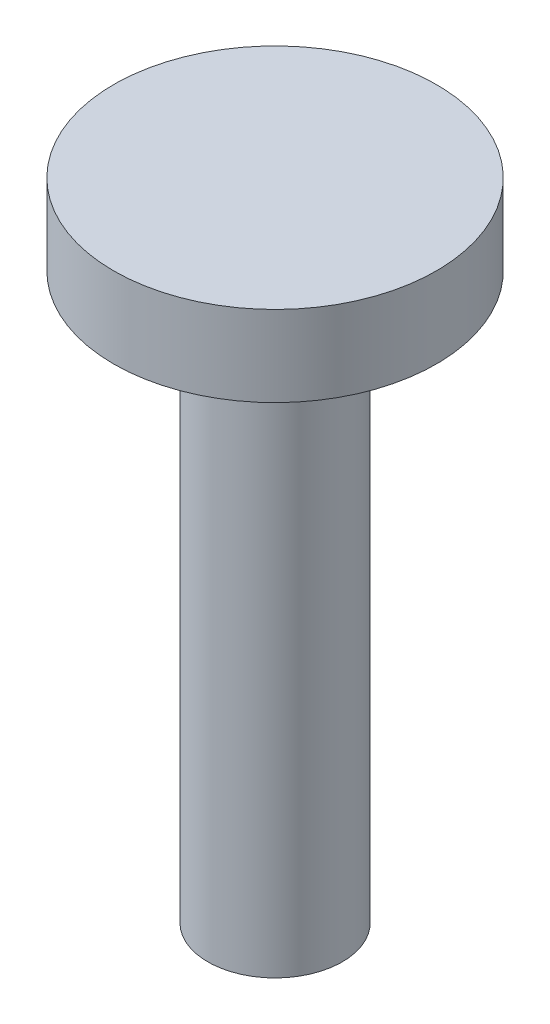
ISO-10303-21;
HEADER;
FILE_DESCRIPTION(('STEP AP214'),'2;1');
FILE_NAME('part.step','',(''),(''),'','','');
FILE_SCHEMA(('AUTOMOTIVE_DESIGN { 1 0 10303 214 1 1 1 1 }'));
ENDSEC;
DATA;
#1=APPLICATION_CONTEXT('core data for automotive mechanical design processes');
#2=APPLICATION_PROTOCOL_DEFINITION('international standard','automotive_design',2000,#1);
#3=PRODUCT_CONTEXT('',#1,'mechanical');
#4=PRODUCT('Part','Part','',(#3));
#5=PRODUCT_RELATED_PRODUCT_CATEGORY('part','',(#4));
#6=PRODUCT_DEFINITION_FORMATION('','',#4);
#7=PRODUCT_DEFINITION_CONTEXT('part definition',#1,'design');
#8=PRODUCT_DEFINITION('design','',#6,#7);
#9=PRODUCT_DEFINITION_SHAPE('','',#8);
#10=(LENGTH_UNIT() NAMED_UNIT(*) SI_UNIT(.MILLI.,.METRE.));
#11=(NAMED_UNIT(*) PLANE_ANGLE_UNIT() SI_UNIT($,.RADIAN.));
#12=(NAMED_UNIT(*) SI_UNIT($,.STERADIAN.) SOLID_ANGLE_UNIT());
#13=UNCERTAINTY_MEASURE_WITH_UNIT(LENGTH_MEASURE(1.E-05),#10,'distance_accuracy_value','');
#14=(GEOMETRIC_REPRESENTATION_CONTEXT(3) GLOBAL_UNCERTAINTY_ASSIGNED_CONTEXT((#13)) GLOBAL_UNIT_ASSIGNED_CONTEXT((#10,
#11,#12)) REPRESENTATION_CONTEXT('',''));
#15=CARTESIAN_POINT('',(0.,0.,0.));
#16=DIRECTION('',(0.,0.,1.));
#17=DIRECTION('',(1.,0.,0.));
#18=AXIS2_PLACEMENT_3D('',#15,#16,#17);
#19=CARTESIAN_POINT('',(0.,10.5,0.));
#20=DIRECTION('',(0.,-1.,0.));
#21=DIRECTION('',(0.,0.,-1.));
#22=AXIS2_PLACEMENT_3D('',#19,#20,#21);
#23=CYLINDRICAL_SURFACE('',#22,2.5);
#24=CARTESIAN_POINT('',(0.,10.5,0.));
#25=DIRECTION('',(0.,1.,0.));
#26=DIRECTION('',(0.,0.,1.));
#27=AXIS2_PLACEMENT_3D('',#24,#25,#26);
#28=CIRCLE('',#27,2.5);
#29=CARTESIAN_POINT('',(0.,10.5,-2.5));
#30=VERTEX_POINT('',#29);
#31=EDGE_CURVE('E10',#30,#30,#28,.T.);
#32=CARTESIAN_POINT('',(0.,-10.5,0.));
#33=DIRECTION('',(0.,1.,0.));
#34=DIRECTION('',(0.,0.,1.));
#35=AXIS2_PLACEMENT_3D('',#32,#33,#34);
#36=CIRCLE('',#35,2.5);
#37=CARTESIAN_POINT('',(0.,-10.5,-2.5));
#38=VERTEX_POINT('',#37);
#39=EDGE_CURVE('E45',#38,#38,#36,.T.);
#40=CARTESIAN_POINT('',(0.,10.5,-2.5));
#41=CARTESIAN_POINT('',(0.,10.28125,-2.5));
#42=CARTESIAN_POINT('',(0.,10.0625,-2.5));
#43=CARTESIAN_POINT('',(0.,9.625,-2.5));
#44=CARTESIAN_POINT('',(0.,9.40625,-2.5));
#45=CARTESIAN_POINT('',(0.,8.96875,-2.5));
#46=CARTESIAN_POINT('',(0.,8.75,-2.5));
#47=CARTESIAN_POINT('',(0.,8.3125,-2.5));
#48=CARTESIAN_POINT('',(0.,8.09375,-2.5));
#49=CARTESIAN_POINT('',(0.,7.65625,-2.5));
#50=CARTESIAN_POINT('',(0.,7.4375,-2.5));
#51=CARTESIAN_POINT('',(0.,7.,-2.5));
#52=CARTESIAN_POINT('',(0.,6.78125,-2.5));
#53=CARTESIAN_POINT('',(0.,6.34375,-2.5));
#54=CARTESIAN_POINT('',(0.,6.125,-2.5));
#55=CARTESIAN_POINT('',(0.,5.6875,-2.5));
#56=CARTESIAN_POINT('',(0.,5.46875,-2.5));
#57=CARTESIAN_POINT('',(0.,5.03125,-2.5));
#58=CARTESIAN_POINT('',(0.,4.8125,-2.5));
#59=CARTESIAN_POINT('',(0.,4.375,-2.5));
#60=CARTESIAN_POINT('',(0.,4.15625,-2.5));
#61=CARTESIAN_POINT('',(0.,3.71875,-2.5));
#62=CARTESIAN_POINT('',(0.,3.5,-2.5));
#63=CARTESIAN_POINT('',(0.,3.0625,-2.5));
#64=CARTESIAN_POINT('',(0.,2.84375,-2.5));
#65=CARTESIAN_POINT('',(0.,2.40625,-2.5));
#66=CARTESIAN_POINT('',(0.,2.1875,-2.5));
#67=CARTESIAN_POINT('',(0.,1.75,-2.5));
#68=CARTESIAN_POINT('',(0.,1.53125,-2.5));
#69=CARTESIAN_POINT('',(0.,1.09375,-2.5));
#70=CARTESIAN_POINT('',(0.,0.875000000000001,-2.5));
#71=CARTESIAN_POINT('',(0.,0.4375,-2.5));
#72=CARTESIAN_POINT('',(0.,0.21875,-2.5));
#73=CARTESIAN_POINT('',(0.,-0.21875,-2.5));
#74=CARTESIAN_POINT('',(0.,-0.4375,-2.5));
#75=CARTESIAN_POINT('',(0.,-0.875000000000001,-2.5));
#76=CARTESIAN_POINT('',(0.,-1.09375,-2.5));
#77=CARTESIAN_POINT('',(0.,-1.53125,-2.5));
#78=CARTESIAN_POINT('',(0.,-1.75,-2.5));
#79=CARTESIAN_POINT('',(0.,-2.1875,-2.5));
#80=CARTESIAN_POINT('',(0.,-2.40625,-2.5));
#81=CARTESIAN_POINT('',(0.,-2.84375,-2.5));
#82=CARTESIAN_POINT('',(0.,-3.0625,-2.5));
#83=CARTESIAN_POINT('',(0.,-3.5,-2.5));
#84=CARTESIAN_POINT('',(0.,-3.71875,-2.5));
#85=CARTESIAN_POINT('',(0.,-4.15625,-2.5));
#86=CARTESIAN_POINT('',(0.,-4.375,-2.5));
#87=CARTESIAN_POINT('',(0.,-4.8125,-2.5));
#88=CARTESIAN_POINT('',(0.,-5.03125,-2.5));
#89=CARTESIAN_POINT('',(0.,-5.46875,-2.5));
#90=CARTESIAN_POINT('',(0.,-5.6875,-2.5));
#91=CARTESIAN_POINT('',(0.,-6.125,-2.5));
#92=CARTESIAN_POINT('',(0.,-6.34375,-2.5));
#93=CARTESIAN_POINT('',(0.,-6.78125,-2.5));
#94=CARTESIAN_POINT('',(0.,-7.,-2.5));
#95=CARTESIAN_POINT('',(0.,-7.4375,-2.5));
#96=CARTESIAN_POINT('',(0.,-7.65625,-2.5));
#97=CARTESIAN_POINT('',(0.,-8.09375,-2.5));
#98=CARTESIAN_POINT('',(0.,-8.3125,-2.5));
#99=CARTESIAN_POINT('',(0.,-8.75,-2.5));
#100=CARTESIAN_POINT('',(0.,-8.96875,-2.5));
#101=CARTESIAN_POINT('',(0.,-9.40625,-2.5));
#102=CARTESIAN_POINT('',(0.,-9.625,-2.5));
#103=CARTESIAN_POINT('',(0.,-10.0625,-2.5));
#104=CARTESIAN_POINT('',(0.,-10.28125,-2.5));
#105=CARTESIAN_POINT('',(0.,-10.5,-2.5));
#106=B_SPLINE_CURVE_WITH_KNOTS('',3,(#40,#41,#42,#43,#44,#45,#46,#47,#48,#49,#50,#51,#52,#53,
#54,#55,#56,#57,#58,#59,#60,#61,#62,#63,#64,#65,#66,#67,#68,#69,#70,#71,#72,#73,#74,#75,#76,#77,
#78,#79,#80,#81,#82,#83,#84,#85,#86,#87,#88,#89,#90,#91,#92,#93,#94,#95,#96,#97,#98,#99,#100,
#101,#102,#103,#104,#105),.UNSPECIFIED.,.F.,.F.,(4,2,2,2,2,2,2,2,2,2,2,2,2,2,2,2,2,2,2,2,2,2,2,
2,2,2,2,2,2,2,2,2,4),(0.,0.656250000000001,1.3125,1.96875,2.625,3.28125,3.9375,4.59375,5.25,
5.90625,6.5625,7.21875,7.875,8.53125,9.1875,9.84375,10.5,11.15625,11.8125,12.46875,13.125,
13.78125,14.4375,15.09375,15.75,16.40625,17.0625,17.71875,18.375,19.03125,19.6875,20.34375,21.),.UNSPECIFIED.);
#107=EDGE_CURVE('BSEAM39',#30,#38,#106,.T.);
#108=ORIENTED_EDGE('',*,*,#31,.F.);
#109=ORIENTED_EDGE('',*,*,#39,.T.);
#110=ORIENTED_EDGE('',*,*,#107,.T.);
#111=ORIENTED_EDGE('',*,*,#107,.F.);
#112=EDGE_LOOP('',(#108,#110,#109,#111));
#113=FACE_BOUND('',#112,.T.);
#114=ADVANCED_FACE('F39',(#113),#23,.T.);
#115=CARTESIAN_POINT('',(0.,-10.5,0.));
#116=DIRECTION('',(0.,1.,0.));
#117=DIRECTION('',(0.,0.,1.));
#118=AXIS2_PLACEMENT_3D('',#115,#116,#117);
#119=PLANE('',#118);
#120=ORIENTED_EDGE('',*,*,#39,.F.);
#121=EDGE_LOOP('',(#120));
#122=FACE_BOUND('',#121,.T.);
#123=ADVANCED_FACE('F61',(#122),#119,.F.);
#124=CARTESIAN_POINT('',(0.,13.5,0.));
#125=DIRECTION('',(0.,-1.,0.));
#126=DIRECTION('',(0.,0.,-1.));
#127=AXIS2_PLACEMENT_3D('',#124,#125,#126);
#128=CYLINDRICAL_SURFACE('',#127,6.);
#129=CARTESIAN_POINT('',(0.,13.5,0.));
#130=DIRECTION('',(0.,1.,0.));
#131=DIRECTION('',(0.,0.,1.));
#132=AXIS2_PLACEMENT_3D('',#129,#130,#131);
#133=CIRCLE('',#132,6.);
#134=CARTESIAN_POINT('',(0.,13.5,6.));
#135=VERTEX_POINT('',#134);
#136=EDGE_CURVE('E47',#135,#135,#133,.T.);
#137=ORIENTED_EDGE('',*,*,#136,.F.);
#138=EDGE_LOOP('',(#137));
#139=FACE_BOUND('',#138,.T.);
#140=CARTESIAN_POINT('',(0.,10.5,0.));
#141=DIRECTION('',(0.,1.,0.));
#142=DIRECTION('',(0.,0.,1.));
#143=AXIS2_PLACEMENT_3D('',#140,#141,#142);
#144=CIRCLE('',#143,6.);
#145=CARTESIAN_POINT('',(0.,10.5,6.));
#146=VERTEX_POINT('',#145);
#147=EDGE_CURVE('E51',#146,#146,#144,.T.);
#148=ORIENTED_EDGE('',*,*,#147,.T.);
#149=EDGE_LOOP('',(#148));
#150=FACE_BOUND('',#149,.T.);
#151=ADVANCED_FACE('F56',(#139,#150),#128,.T.);
#152=CARTESIAN_POINT('',(0.,13.5,0.));
#153=DIRECTION('',(0.,1.,0.));
#154=DIRECTION('',(0.,0.,1.));
#155=AXIS2_PLACEMENT_3D('',#152,#153,#154);
#156=PLANE('',#155);
#157=ORIENTED_EDGE('',*,*,#136,.T.);
#158=EDGE_LOOP('',(#157));
#159=FACE_BOUND('',#158,.T.);
#160=ADVANCED_FACE('F60',(#159),#156,.T.);
#161=CARTESIAN_POINT('',(0.,10.5,0.));
#162=DIRECTION('',(0.,1.,0.));
#163=DIRECTION('',(0.,0.,1.));
#164=AXIS2_PLACEMENT_3D('',#161,#162,#163);
#165=PLANE('',#164);
#166=ORIENTED_EDGE('',*,*,#31,.T.);
#167=EDGE_LOOP('',(#166));
#168=FACE_BOUND('',#167,.T.);
#169=ORIENTED_EDGE('',*,*,#147,.F.);
#170=EDGE_LOOP('',(#169));
#171=FACE_BOUND('',#170,.T.);
#172=ADVANCED_FACE('F66',(#168,#171),#165,.F.);
#173=CLOSED_SHELL('',(#114,#123,#151,#160,#172));
#174=MANIFOLD_SOLID_BREP('B2',#173);
#175=ADVANCED_BREP_SHAPE_REPRESENTATION('',(#18,#174),#14);
#176=SHAPE_DEFINITION_REPRESENTATION(#9,#175);
ENDSEC;
END-ISO-10303-21;
